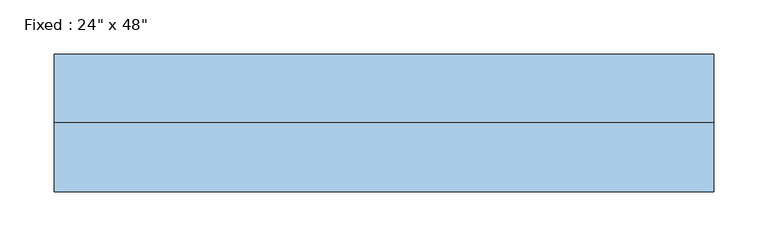
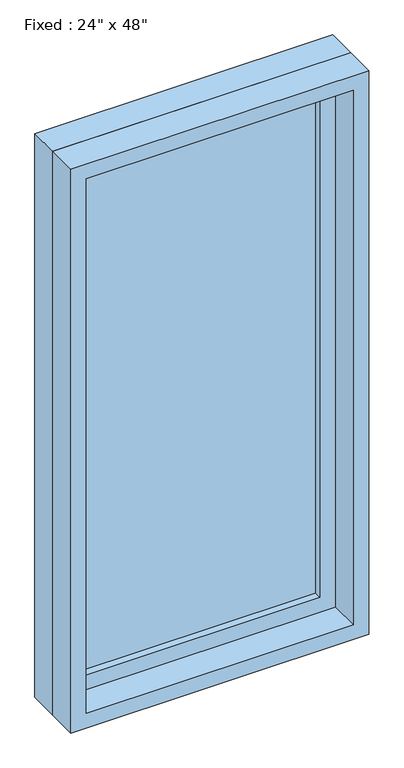
"""IFC4 building model written with IfcOpenShell, lengths in millimetres: window geometry."""

from ifc_helpers import new_model, si_unit, frame, origin, place, context, project, spatial, polyline, outline, extrude, source, transform, mapped, element, save


def window_4879aceb(model_context):
    return source(origin(), model_context, "Body", "SweptSolid", [
        extrude(outline(polyline([(203.2, 15.875), (-279.4, 15.875), (-279.4, 28.575), (203.2, 28.575), (203.2, 15.875)])), frame((0.0, 0.0, 977.9), z_axis=(0.0, 0.0, 1.0), x_axis=(1.0, 0.0, 0.0)), (0.0, 0.0, 1.0), 1092.2),
        extrude(outline(polyline([(2114.55, -323.85), (933.45, -323.85), (933.45, 247.65), (2114.55, 247.65), (2114.55, -323.85)]), holes=[polyline([(2070.1, -279.4), (2070.1, 203.2), (977.9, 203.2), (977.9, -279.4), (2070.1, -279.4)])]), frame((0.0, 0.0, 0.0), z_axis=(0.0, 1.0, 0.0), x_axis=(0.0, 0.0, 1.0)), (0.0, 0.0, 1.0), 44.45),
        extrude(outline(polyline([(2133.6, -342.9), (914.4, -342.9), (914.4, 266.7), (2133.6, 266.7), (2133.6, -342.9)]), holes=[polyline([(2101.85, -311.15), (2101.85, 234.95), (946.15, 234.95), (946.15, -311.15), (2101.85, -311.15)])]), frame((0.0, -63.5, 0.0), z_axis=(0.0, 1.0, 0.0), x_axis=(0.0, 0.0, 1.0)), (0.0, 0.0, 1.0), 63.5),
        extrude(outline(polyline([(2133.6, 266.7), (2133.6, -342.9), (914.4, -342.9), (914.4, 266.7), (2133.6, 266.7)]), holes=[polyline([(2114.55, 247.65), (933.45, 247.65), (933.45, -323.85), (2114.55, -323.85), (2114.55, 247.65)])]), frame((0.0, 0.0, 0.0), z_axis=(0.0, 1.0, 0.0), x_axis=(0.0, 0.0, 1.0)), (0.0, 0.0, 1.0), 63.5),
    ])


if __name__ == "__main__":
    model = new_model("IFC4")
    model_context = context("Model", 3, world=origin())
    ifc_project = project(units=[si_unit("LENGTHUNIT", "METRE", prefix="MILLI")], contexts=[model_context])
    site = spatial("IfcSite", under=ifc_project)
    building = spatial("IfcBuilding", under=site)
    placement = place(None, origin())
    window_shape = window_4879aceb(model_context)
    element("IfcWindow", 1, ObjectType="Fixed : 24\" x 48\"", at=placement, inside=building, context=model_context, shape_type="MappedRepresentation", body=[
        mapped(window_shape, transform((0.0, 0.0, 0.0), x_axis=(1.0, 0.0, 0.0), y_axis=(0.0, 1.0, 0.0), z_axis=(0.0, 0.0, 1.0))),
    ])
    save(model, "model.ifc")

# Revit data of these elements
# Type "Fixed : 24\" x 48\""
#   Type Mark = "2"
#   Construction Type Id = "GSP4R"
#   Assembly Code = "B2020100"
#   Analytic Construction = "1/8 in Pilkington single glazing"
#   Visual Light Transmittance = 0.9
#   Solar Heat Gain Coefficient = 0.78
#   Heat Transfer Coefficient (U) = 0.6496 BTU/(h·ft²·°F)
#   Height = 4' - 0"
#   Default Sill Height = 3' - 0"
#   Width = 2' - 0"
#   Window Inset = 0' - 0 3/4"
#   Define Thermal Properties by = 1
#   Glass Pane Material = Glass
#   Sash Material = Sash
#   Wall Closure = (empty or 0)
# Element 1 (IfcWindow, "Fixed : 24\" x 48\"")
#   Materials on its faces: "Sash", "Glass"
# Materials
#   "Glass": class "Glass", colour RGB 0 128 192, transparency 0.75, Description = "Soda Lime Glass", Cost = 0
#   "Sash": class "Wood", colour RGB 224 178 126, transparency 0
